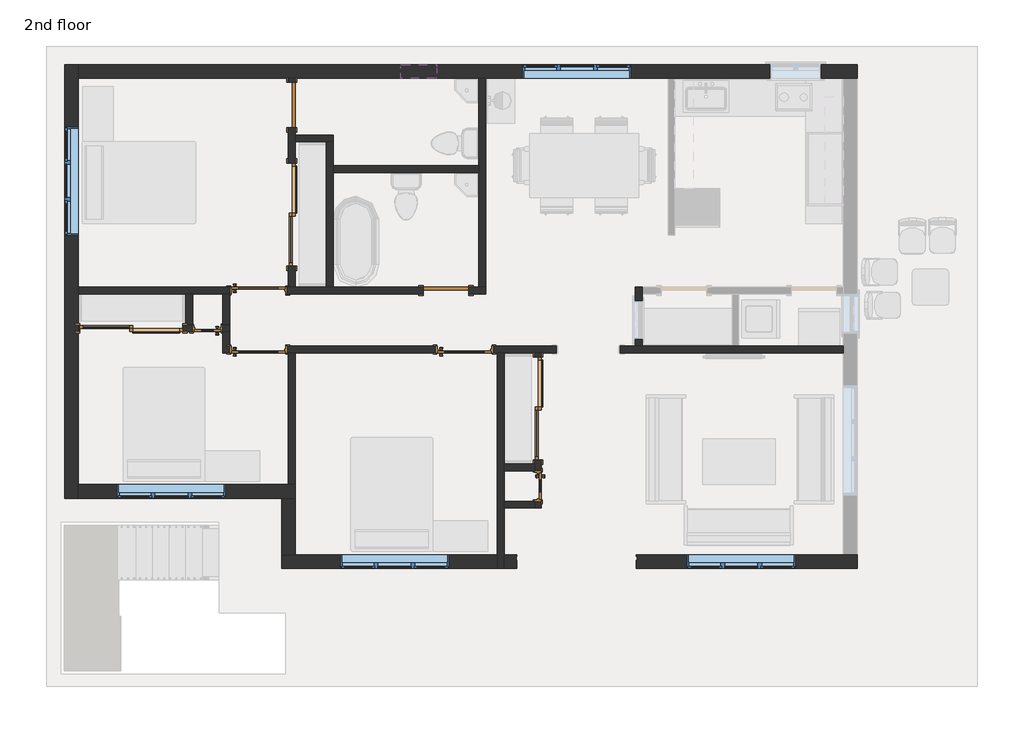
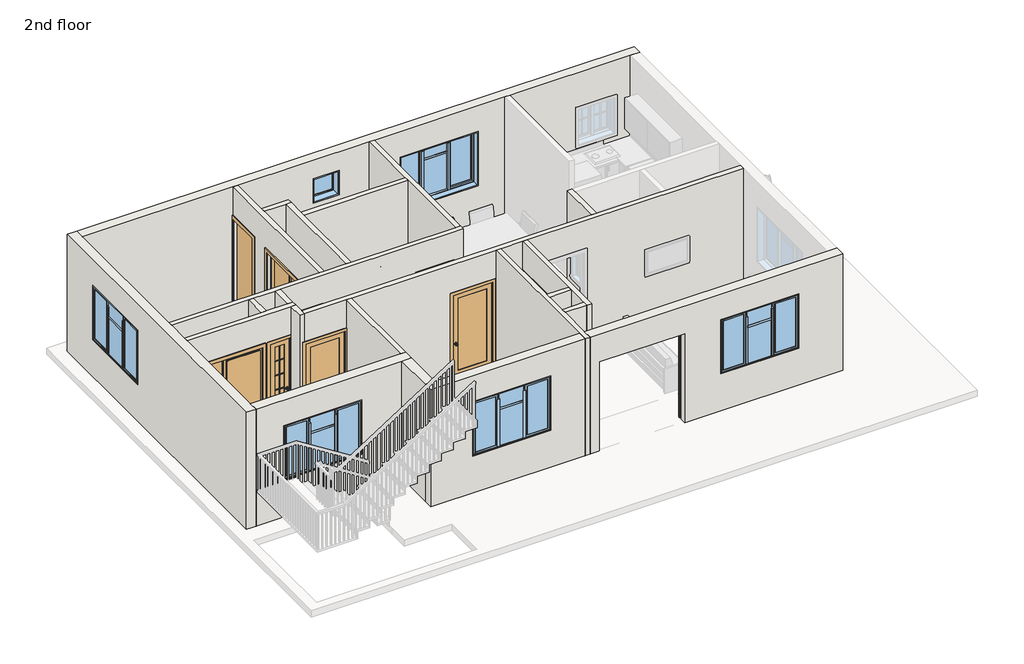
# One storey, part 1 of 4: 23 walls, 10 doors, 6 windows.
"""IFC4 building model written with IfcOpenShell, lengths in millimetres."""

from ifc_helpers import new_model, si_unit, frame, origin, place, context, project, spatial, polyline, outline, extrude, faceted_brep, transform, mapped, element, save
from components import door_505787c2, door_a3feeac7, door_3c6ab76a, door_ccf0cbd1, door_214872d5, door_78caadf7, window_80340324, window_7a1f68bc

model = new_model("IFC4")

# Units and contexts
model_context = context("Model", 3, world=origin())
ifc_project = project(units=[si_unit("LENGTHUNIT", "METRE", prefix="MILLI")], contexts=[model_context])

# Site, building, storey
site = spatial("IfcSite", under=ifc_project)
building = spatial("IfcBuilding", under=site)
storey = spatial("IfcBuildingStorey", under=building, Name="2nd floor", Elevation=7010.4)

# Doors
placement = place(None, origin())
door_shape = door_505787c2(model_context)
element("IfcDoor", 1, ObjectType="Door-Double-Sliding : 68\" x 84\"", at=placement, inside=storey, context=model_context, shape_type="MappedRepresentation", body=[
    mapped(door_shape, transform((-1350.0263529, 910.5161978, 7010.4), x_axis=(0.0, -1.0, 0.0), y_axis=(1.0, 0.0, 0.0), z_axis=(0.0, 0.0, 1.0))),
])
element("IfcDoor", 2, ObjectType="Door-Double-Sliding : 68\" x 84\"", at=placement, inside=storey, context=model_context, shape_type="MappedRepresentation", body=[
    mapped(door_shape, transform((-8046.1013529, 2383.7161978, 7010.4), x_axis=(-1.0, 0.0, 0.0), y_axis=(0.0, -1.0, 0.0), z_axis=(0.0, 0.0, 1.0))),
])
element("IfcDoor", 3, ObjectType="Door-Double-Sliding : 68\" x 84\"", at=placement, inside=storey, context=model_context, shape_type="MappedRepresentation", body=[
    mapped(door_shape, transform((-5477.5263529, 4168.0661978, 7010.4), x_axis=(0.0, -1.0, 0.0), y_axis=(1.0, 0.0, 0.0), z_axis=(0.0, 0.0, 1.0))),
])
door_2_shape = door_a3feeac7(model_context)
element("IfcDoor", 4, ObjectType="Door-Interior-Single-1_Panel-Wood : 36\" x 84\"", at=placement, inside=storey, context=model_context, shape_type="MappedRepresentation", body=[
    mapped(door_2_shape, transform((-5912.5013529, 1897.9411978, 7010.4), x_axis=(1.0, 0.0, 0.0), y_axis=(0.0, 1.0, 0.0), z_axis=(0.0, 0.0, 1.0))),
])
element("IfcDoor", 5, ObjectType="Door-Interior-Single-1_Panel-Wood : 36\" x 84\"", at=placement, inside=storey, context=model_context, shape_type="MappedRepresentation", body=[
    mapped(door_2_shape, transform((-2454.9263529, 1897.9411978, 7010.4), x_axis=(1.0, 0.0, 0.0), y_axis=(0.0, 1.0, 0.0), z_axis=(0.0, 0.0, 1.0))),
])
door_3_shape = door_3c6ab76a(model_context)
element("IfcDoor", 6, ObjectType="Door-Interior-Single-1_Panel-Wood : 36\" x 84\"", at=placement, inside=storey, context=model_context, shape_type="MappedRepresentation", body=[
    mapped(door_3_shape, transform((-5912.5013529, 2894.8911978, 7010.4), x_axis=(1.0, 0.0, 0.0), y_axis=(0.0, 1.0, 0.0), z_axis=(0.0, 0.0, 1.0))),
])
door_4_shape = door_ccf0cbd1(model_context)
element("IfcDoor", 7, ObjectType="Door-Interior-Single-Full Glass-Wood : 18\" x 84\"", at=placement, inside=storey, context=model_context, shape_type="MappedRepresentation", body=[
    mapped(door_4_shape, transform((-1219.8513529, -391.2338022, 7010.4), x_axis=(0.0, -1.0, 0.0), y_axis=(1.0, 0.0, 0.0), z_axis=(0.0, 0.0, 1.0))),
])
element("IfcDoor", 8, ObjectType="Door-Interior-Single-Full Glass-Wood : 18\" x 84\"", at=placement, inside=storey, context=model_context, shape_type="MappedRepresentation", body=[
    mapped(door_4_shape, transform((-6766.5763529, 2253.5411978, 7010.4), x_axis=(-1.0, 0.0, 0.0), y_axis=(0.0, -1.0, 0.0), z_axis=(0.0, 0.0, 1.0))),
])
door_5_shape = door_214872d5(model_context)
element("IfcDoor", 9, ObjectType="Single-Flush : 30\" x 84\"", at=placement, inside=storey, context=model_context, shape_type="MappedRepresentation", body=[
    mapped(door_5_shape, transform((-2766.0763529, 2891.7161978, 7010.4), x_axis=(1.0, 0.0, 0.0), y_axis=(0.0, 1.0, 0.0), z_axis=(0.0, 0.0, 1.0))),
])
door_6_shape = door_78caadf7(model_context)
element("IfcDoor", 10, ObjectType="Single-Flush : 30\" x 84\"", at=placement, inside=storey, context=model_context, shape_type="MappedRepresentation", body=[
    mapped(door_6_shape, transform((-5350.5263529, 6006.3911978, 7010.4), x_axis=(0.0, 1.0, 0.0), y_axis=(-1.0, 0.0, 0.0), z_axis=(0.0, 0.0, 1.0))),
])

# Walls
element("IfcWall", 11, ObjectType="Generic - 4.5\"", at=placement, inside=storey, context=model_context, shape_type="Brep", body=[
    faceted_brep([(-5407.6763529, 6454.0661978, 7010.4), (-5407.6763529, 6387.3911978, 7010.4), (-5407.6763529, 6387.3911978, 9144.0), (-5407.6763529, 5625.3911978, 9144.0), (-5407.6763529, 5625.3911978, 7010.4), (-5407.6763529, 5031.6661978, 7010.4), (-5407.6763529, 5031.6661978, 9144.0), (-5407.6763529, 3304.4661978, 9144.0), (-5407.6763529, 3304.4661978, 7010.4), (-5407.6763529, 2948.8661978, 7010.4), (-5407.6763529, 2948.8661978, 9906.0), (-5407.6763529, 6454.0661978, 9906.0), (-5293.3763529, 6387.3911978, 9144.0), (-5293.3763529, 6387.3911978, 7010.4), (-5293.3763529, 6454.0661978, 7010.4), (-5293.3763529, 6454.0661978, 9906.0), (-5293.3763529, 5501.5661978, 9906.0), (-5293.3763529, 5387.2661978, 9906.0), (-5293.3763529, 2948.8661978, 9906.0), (-5293.3763529, 2948.8661978, 7010.4), (-5293.3763529, 3304.4661978, 7010.4), (-5293.3763529, 3304.4661978, 9144.0), (-5293.3763529, 5031.6661978, 9144.0), (-5293.3763529, 5031.6661978, 7010.4), (-5293.3763529, 5387.2661978, 7010.4), (-5293.3763529, 5501.5661978, 7010.4), (-5293.3763529, 5625.3911978, 7010.4), (-5293.3763529, 5625.3911978, 9144.0)], [[[0, 1, 2, 3, 4, 5, 6, 7, 8, 9, 10, 11]], [[12, 13, 14, 15, 16, 17, 18, 19, 20, 21, 22, 23, 24, 25, 26, 27]], [[9, 8, 20, 19]], [[14, 13, 1, 0]], [[26, 25, 24, 23, 5, 4]], [[11, 10, 18, 17, 16, 15]], [[0, 11, 15, 14]], [[10, 9, 19, 18]], [[23, 22, 6, 5]], [[21, 20, 8, 7]], [[22, 21, 7, 6]], [[2, 1, 13, 12]], [[3, 2, 12, 27]], [[4, 3, 27, 26]]]),
])
element("IfcWall", 12, ObjectType="Generic - 4.5\"", at=placement, inside=storey, context=model_context, shape_type="Brep", body=[
    faceted_brep([(-2099.3263529, 2948.8661978, 7010.4), (-2213.6263529, 2948.8661978, 7010.4), (-2385.0763529, 2948.8661978, 7010.4), (-2385.0763529, 2948.8661978, 9144.0), (-3147.0763529, 2948.8661978, 9144.0), (-3147.0763529, 2948.8661978, 7010.4), (-4658.3763529, 2948.8661978, 7010.4), (-4772.6763529, 2948.8661978, 7010.4), (-5293.3763529, 2948.8661978, 7010.4), (-5407.6763529, 2948.8661978, 7010.4), (-5429.9013529, 2948.8661978, 7010.4), (-5429.9013529, 2948.8661978, 9169.4), (-6395.1013529, 2948.8661978, 9169.4), (-6395.1013529, 2948.8661978, 7010.4), (-8931.9263529, 2948.8661978, 7010.4), (-8931.9263529, 2948.8661978, 9906.0), (-5407.6763529, 2948.8661978, 9906.0), (-5293.3763529, 2948.8661978, 9906.0), (-4772.6763529, 2948.8661978, 9906.0), (-4658.3763529, 2948.8661978, 9906.0), (-2213.6263529, 2948.8661978, 9906.0), (-2099.3263529, 2948.8661978, 9906.0), (-2385.0763529, 2834.5661978, 9144.0), (-2385.0763529, 2834.5661978, 7010.4), (-2099.3263529, 2834.5661978, 7010.4), (-2099.3263529, 2834.5661978, 9906.0), (-6391.9263529, 2834.5661978, 9906.0), (-6506.2263529, 2834.5661978, 9906.0), (-7014.2263529, 2834.5661978, 9906.0), (-7128.5263529, 2834.5661978, 9906.0), (-8931.9263529, 2834.5661978, 9906.0), (-8931.9263529, 2834.5661978, 7010.4), (-7128.5263529, 2834.5661978, 7010.4), (-7014.2263529, 2834.5661978, 7010.4), (-6506.2263529, 2834.5661978, 7010.4), (-6395.1013529, 2834.5661978, 7010.4), (-6395.1013529, 2834.5661978, 9169.4), (-5429.9013529, 2834.5661978, 9169.4), (-5429.9013529, 2834.5661978, 7010.4), (-3147.0763529, 2834.5661978, 7010.4), (-3147.0763529, 2834.5661978, 9144.0)], [[[0, 1, 2, 3, 4, 5, 6, 7, 8, 9, 10, 11, 12, 13, 14, 15, 16, 17, 18, 19, 20, 21]], [[22, 23, 24, 25, 26, 27, 28, 29, 30, 31, 32, 33, 34, 35, 36, 37, 38, 39, 40]], [[31, 14, 13, 35, 34, 33, 32]], [[39, 38, 10, 9, 8, 7, 6, 5]], [[24, 23, 2, 1, 0]], [[21, 20, 19, 18, 17, 16, 15, 30, 29, 28, 27, 26, 25]], [[15, 14, 31, 30]], [[0, 21, 25, 24]], [[37, 11, 10, 38]], [[11, 37, 36, 12]], [[12, 36, 35, 13]], [[3, 2, 23, 22]], [[4, 3, 22, 40]], [[5, 4, 40, 39]]]),
])
element("IfcWall", 13, ObjectType="Generic - 4.5\"", at=placement, inside=storey, context=model_context, shape_type="Brep", body=[
    faceted_brep([(-8931.9263529, 2199.5661978, 7010.4), (-8909.7013529, 2199.5661978, 7010.4), (-8909.7013529, 2199.5661978, 9144.0), (-7182.5013529, 2199.5661978, 9144.0), (-7182.5013529, 2199.5661978, 7010.4), (-7020.5763529, 2199.5661978, 7010.4), (-7020.5763529, 2199.5661978, 9169.4), (-6512.5763529, 2199.5661978, 9169.4), (-6512.5763529, 2199.5661978, 7010.4), (-6506.2263529, 2199.5661978, 7010.4), (-6391.9263529, 2199.5661978, 7010.4), (-6391.9263529, 2199.5661978, 9906.0), (-6506.2263529, 2199.5661978, 9906.0), (-8931.9263529, 2199.5661978, 9906.0), (-8909.7013529, 2313.8661978, 9144.0), (-8909.7013529, 2313.8661978, 7010.4), (-8931.9263529, 2313.8661978, 7010.4), (-8931.9263529, 2313.8661978, 9906.0), (-7128.5263529, 2313.8661978, 9906.0), (-7014.2263529, 2313.8661978, 9906.0), (-6506.2263529, 2313.8661978, 9906.0), (-6391.9263529, 2313.8661978, 9906.0), (-6391.9263529, 2313.8661978, 7010.4), (-6506.2263529, 2313.8661978, 7010.4), (-6512.5763529, 2313.8661978, 7010.4), (-6512.5763529, 2313.8661978, 9169.4), (-7020.5763529, 2313.8661978, 9169.4), (-7020.5763529, 2313.8661978, 7010.4), (-7128.5263529, 2313.8661978, 7010.4), (-7182.5013529, 2313.8661978, 7010.4), (-7182.5013529, 2313.8661978, 9144.0)], [[[0, 1, 2, 3, 4, 5, 6, 7, 8, 9, 10, 11, 12, 13]], [[14, 15, 16, 17, 18, 19, 20, 21, 22, 23, 24, 25, 26, 27, 28, 29, 30]], [[22, 10, 9, 8, 24, 23]], [[16, 15, 1, 0]], [[29, 28, 27, 5, 4]], [[13, 12, 11, 21, 20, 19, 18, 17]], [[0, 13, 17, 16]], [[11, 10, 22, 21]], [[26, 6, 5, 27]], [[6, 26, 25, 7]], [[7, 25, 24, 8]], [[4, 3, 30, 29]], [[2, 1, 15, 14]], [[3, 2, 14, 30]]]),
])
element("IfcWall", 14, ObjectType="Generic - 4.5\"", at=placement, inside=storey, context=model_context, shape_type="Brep", body=[
    faceted_brep([(-7014.2263529, 2313.8661978, 7010.4), (-7014.2263529, 2834.5661978, 7010.4), (-7014.2263529, 2834.5661978, 9906.0), (-7014.2263529, 2313.8661978, 9906.0), (-7128.5263529, 2313.8661978, 7010.4), (-7128.5263529, 2313.8661978, 9906.0), (-7128.5263529, 2834.5661978, 9906.0), (-7128.5263529, 2834.5661978, 7010.4), (-7020.5763529, 2313.8661978, 7010.4)], [[[0, 1, 2, 3]], [[4, 5, 6, 7]], [[1, 0, 8, 4, 7]], [[3, 2, 6, 5]], [[0, 3, 5, 4, 8]], [[2, 1, 7, 6]]]),
])
element("IfcWall", 15, ObjectType="Generic - 4.5\"", at=placement, inside=storey, context=model_context, shape_type="Brep", body=[
    faceted_brep([(-6391.9263529, 2313.8661978, 7010.4), (-6391.9263529, 2834.5661978, 7010.4), (-6391.9263529, 2834.5661978, 9906.0), (-6391.9263529, 2313.8661978, 9906.0), (-6506.2263529, 2313.8661978, 7010.4), (-6506.2263529, 2313.8661978, 9906.0), (-6506.2263529, 2834.5661978, 9906.0), (-6506.2263529, 2834.5661978, 7010.4), (-6395.1013529, 2834.5661978, 7010.4)], [[[0, 1, 2, 3]], [[4, 5, 6, 7]], [[1, 0, 4, 7, 8]], [[3, 2, 6, 5]], [[0, 3, 5, 4]], [[2, 1, 8, 7, 6]]]),
])
element("IfcWall", 16, ObjectType="Generic - 4.5\"", at=placement, inside=storey, context=model_context, shape_type="SweptSolid", body=[
    extrude(outline(polyline([(-5293.3763529, 1843.9661978), (-5293.3763529, -365.8338022), (-5407.6763529, -365.8338022), (-5407.6763529, 1843.9661978), (-5293.3763529, 1843.9661978)])), frame((0.0, 0.0, 7010.4), z_axis=(0.0, 0.0, 1.0), x_axis=(1.0, 0.0, 0.0)), (0.0, 0.0, 1.0), 2895.6),
])
element("IfcWall", 17, ObjectType="Generic - 4.5\"", at=placement, inside=storey, context=model_context, shape_type="Brep", body=[
    faceted_brep([(-6506.2263529, 2199.5661978, 7010.4), (-6506.2263529, 1843.9661978, 7010.4), (-6506.2263529, 1843.9661978, 9906.0), (-6506.2263529, 2199.5661978, 9906.0), (-6391.9263529, 2199.5661978, 9906.0), (-6391.9263529, 1958.2661978, 9906.0), (-6391.9263529, 1843.9661978, 9906.0), (-6391.9263529, 1843.9661978, 9169.4), (-6391.9263529, 1958.2661978, 9169.4), (-6391.9263529, 1958.2661978, 7010.4), (-6391.9263529, 2199.5661978, 7010.4), (-6395.1013529, 1958.2661978, 7010.4), (-6395.1013529, 1843.9661978, 7010.4), (-6395.1013529, 1843.9661978, 9169.4), (-6395.1013529, 1958.2661978, 9169.4)], [[[0, 1, 2, 3]], [[4, 5, 6, 7, 8, 9, 10]], [[1, 0, 10, 9, 11, 12]], [[3, 2, 6, 5, 4]], [[0, 3, 4, 10]], [[2, 1, 12, 13, 7, 6]], [[14, 11, 9, 8]], [[13, 14, 8, 7]], [[11, 14, 13, 12]]]),
])
element("IfcWall", 18, ObjectType="Generic - 4.5\"", at=placement, inside=storey, context=model_context, shape_type="Brep", body=[
    faceted_brep([(-1972.3263529, 1843.9661978, 7010.4), (-1902.4763529, 1843.9661978, 7010.4), (-1788.1763529, 1843.9661978, 7010.4), (-1280.1763529, 1843.9661978, 7010.4), (-1165.8763529, 1843.9661978, 7010.4), (-911.8763529, 1843.9661978, 7010.4), (-911.8763529, 1843.9661978, 9144.0), (154.9236471, 1843.9661978, 9144.0), (154.9236471, 1843.9661978, 7010.4), (3901.4236471, 1843.9661978, 7010.4), (3901.4236471, 1843.9661978, 9906.0), (-1165.8763529, 1843.9661978, 9906.0), (-1280.1763529, 1843.9661978, 9906.0), (-1788.1763529, 1843.9661978, 9906.0), (-1902.4763529, 1843.9661978, 9906.0), (-5293.3763529, 1843.9661978, 9906.0), (-5407.6763529, 1843.9661978, 9906.0), (-6391.9263529, 1843.9661978, 9906.0), (-6391.9263529, 1843.9661978, 9169.4), (-5429.9013529, 1843.9661978, 9169.4), (-5429.9013529, 1843.9661978, 7010.4), (-5407.6763529, 1843.9661978, 7010.4), (-5293.3763529, 1843.9661978, 7010.4), (-2937.5263529, 1843.9661978, 7010.4), (-2937.5263529, 1843.9661978, 9169.4), (-1972.3263529, 1843.9661978, 9169.4), (-911.8763529, 1958.2661978, 9144.0), (-911.8763529, 1958.2661978, 7010.4), (-1972.3263529, 1958.2661978, 7010.4), (-1972.3263529, 1958.2661978, 9169.4), (-2937.5263529, 1958.2661978, 9169.4), (-2937.5263529, 1958.2661978, 7010.4), (-5429.9013529, 1958.2661978, 7010.4), (-5429.9013529, 1958.2661978, 9169.4), (-6391.9263529, 1958.2661978, 9169.4), (-6391.9263529, 1958.2661978, 9906.0), (408.9236471, 1958.2661978, 9906.0), (523.2236471, 1958.2661978, 9906.0), (2034.5236471, 1958.2661978, 9906.0), (2148.8236471, 1958.2661978, 9906.0), (3901.4236471, 1958.2661978, 9906.0), (3901.4236471, 1958.2661978, 7010.4), (2148.8236471, 1958.2661978, 7010.4), (2034.5236471, 1958.2661978, 7010.4), (523.2236471, 1958.2661978, 7010.4), (408.9236471, 1958.2661978, 7010.4), (154.9236471, 1958.2661978, 7010.4), (154.9236471, 1958.2661978, 9144.0)], [[[0, 1, 2, 3, 4, 5, 6, 7, 8, 9, 10, 11, 12, 13, 14, 15, 16, 17, 18, 19, 20, 21, 22, 23, 24, 25]], [[26, 27, 28, 29, 30, 31, 32, 33, 34, 35, 36, 37, 38, 39, 40, 41, 42, 43, 44, 45, 46, 47]], [[20, 32, 31, 23, 22, 21]], [[28, 27, 5, 4, 3, 2, 1, 0]], [[46, 45, 44, 43, 42, 41, 9, 8]], [[17, 16, 15, 14, 13, 12, 11, 10, 40, 39, 38, 37, 36, 35]], [[17, 35, 34, 18]], [[10, 9, 41, 40]], [[19, 18, 34, 33]], [[25, 29, 28, 0]], [[29, 25, 24, 30]], [[30, 24, 23, 31]], [[19, 33, 32, 20]], [[8, 7, 47, 46]], [[6, 5, 27, 26]], [[7, 6, 26, 47]]]),
])
element("IfcWall", 19, ObjectType="Generic - 4.5\"", at=placement, inside=storey, context=model_context, shape_type="Brep", body=[
    faceted_brep([(-1902.4763529, 1843.9661978, 7010.4), (-1902.4763529, -1546.9338022, 7010.4), (-1902.4763529, -1775.5338022, 7010.4), (-1902.4763529, -1775.5338022, 9906.0), (-1902.4763529, -1546.9338022, 9906.0), (-1902.4763529, 1843.9661978, 9906.0), (-1788.1763529, 1843.9661978, 7010.4), (-1788.1763529, 1843.9661978, 9906.0), (-1788.1763529, -22.9338022, 9906.0), (-1788.1763529, -137.2338022, 9906.0), (-1788.1763529, -645.2338022, 9906.0), (-1788.1763529, -759.5338022, 9906.0), (-1788.1763529, -1546.9338022, 9906.0), (-1788.1763529, -1775.5338022, 9906.0), (-1788.1763529, -1775.5338022, 7010.4), (-1788.1763529, -1546.9338022, 7010.4), (-1788.1763529, -759.5338022, 7010.4), (-1788.1763529, -645.2338022, 7010.4), (-1788.1763529, -137.2338022, 7010.4), (-1788.1763529, -22.9338022, 7010.4)], [[[0, 1, 2, 3, 4, 5]], [[6, 7, 8, 9, 10, 11, 12, 13, 14, 15, 16, 17, 18, 19]], [[2, 1, 0, 6, 19, 18, 17, 16, 15, 14]], [[5, 4, 3, 13, 12, 11, 10, 9, 8, 7]], [[0, 5, 7, 6]], [[3, 2, 14, 13]]]),
])
element("IfcWall", 20, ObjectType="Generic - 4.5\"", at=placement, inside=storey, context=model_context, shape_type="Brep", body=[
    faceted_brep([(-1280.1763529, 46.9161978, 9144.0), (-1280.1763529, 46.9161978, 7010.4), (-1280.1763529, -22.9338022, 7010.4), (-1280.1763529, -137.2338022, 7010.4), (-1280.1763529, -137.2338022, 9169.4), (-1280.1763529, -645.2338022, 9169.4), (-1280.1763529, -645.2338022, 7010.4), (-1280.1763529, -759.5338022, 7010.4), (-1280.1763529, -759.5338022, 9906.0), (-1280.1763529, -645.2338022, 9906.0), (-1280.1763529, -137.2338022, 9906.0), (-1280.1763529, -22.9338022, 9906.0), (-1280.1763529, 1843.9661978, 9906.0), (-1280.1763529, 1843.9661978, 7010.4), (-1280.1763529, 1774.1161978, 7010.4), (-1280.1763529, 1774.1161978, 9144.0), (-1165.8763529, -137.2338022, 7010.4), (-1165.8763529, 46.9161978, 7010.4), (-1165.8763529, 46.9161978, 9144.0), (-1165.8763529, 1774.1161978, 9144.0), (-1165.8763529, 1774.1161978, 7010.4), (-1165.8763529, 1843.9661978, 7010.4), (-1165.8763529, 1843.9661978, 9906.0), (-1165.8763529, -759.5338022, 9906.0), (-1165.8763529, -759.5338022, 7010.4), (-1165.8763529, -645.2338022, 7010.4), (-1165.8763529, -645.2338022, 9169.4), (-1165.8763529, -137.2338022, 9169.4)], [[[0, 1, 2, 3, 4, 5, 6, 7, 8, 9, 10, 11, 12, 13, 14, 15]], [[16, 17, 18, 19, 20, 21, 22, 23, 24, 25, 26, 27]], [[24, 7, 6, 25]], [[14, 13, 21, 20]], [[3, 2, 1, 17, 16]], [[12, 11, 10, 9, 8, 23, 22]], [[13, 12, 22, 21]], [[8, 7, 24, 23]], [[5, 26, 25, 6]], [[26, 5, 4, 27]], [[27, 4, 3, 16]], [[20, 19, 15, 14]], [[18, 17, 1, 0]], [[19, 18, 0, 15]]]),
])
element("IfcWall", 21, ObjectType="Generic - 4.5\"", at=placement, inside=storey, context=model_context, shape_type="Brep", body=[
    faceted_brep([(-1280.1763529, -22.9338022, 7010.4), (-1788.1763529, -22.9338022, 7010.4), (-1788.1763529, -22.9338022, 9906.0), (-1280.1763529, -22.9338022, 9906.0), (-1280.1763529, -137.2338022, 7010.4), (-1280.1763529, -137.2338022, 9169.4), (-1280.1763529, -137.2338022, 9906.0), (-1788.1763529, -137.2338022, 9906.0), (-1788.1763529, -137.2338022, 7010.4)], [[[0, 1, 2, 3]], [[4, 5, 6, 7, 8]], [[1, 0, 4, 8]], [[3, 2, 7, 6]], [[0, 3, 6, 5, 4]], [[2, 1, 8, 7]]]),
])
element("IfcWall", 22, ObjectType="Generic - 4.5\"", at=placement, inside=storey, context=model_context, shape_type="Brep", body=[
    faceted_brep([(-1280.1763529, -645.2338022, 7010.4), (-1788.1763529, -645.2338022, 7010.4), (-1788.1763529, -645.2338022, 9906.0), (-1280.1763529, -645.2338022, 9906.0), (-1280.1763529, -645.2338022, 9169.4), (-1280.1763529, -759.5338022, 7010.4), (-1280.1763529, -759.5338022, 9906.0), (-1788.1763529, -759.5338022, 9906.0), (-1788.1763529, -759.5338022, 7010.4)], [[[0, 1, 2, 3, 4]], [[5, 6, 7, 8]], [[1, 0, 5, 8]], [[3, 2, 7, 6]], [[0, 4, 3, 6, 5]], [[2, 1, 8, 7]]]),
])
element("IfcWall", 23, ObjectType="Generic - 4.5\"", at=placement, inside=storey, context=model_context, shape_type="Brep", body=[
    faceted_brep([(-2099.3263529, 2948.8661978, 7010.4), (-2099.3263529, 6454.0661978, 7010.4), (-2099.3263529, 6454.0661978, 9906.0), (-2099.3263529, 2948.8661978, 9906.0), (-2213.6263529, 2948.8661978, 7010.4), (-2213.6263529, 2948.8661978, 9906.0), (-2213.6263529, 4872.9161978, 9906.0), (-2213.6263529, 4987.2161978, 9906.0), (-2213.6263529, 6454.0661978, 9906.0), (-2213.6263529, 6454.0661978, 7010.4), (-2213.6263529, 4987.2161978, 7010.4), (-2213.6263529, 4872.9161978, 7010.4)], [[[0, 1, 2, 3]], [[4, 5, 6, 7, 8, 9, 10, 11]], [[1, 0, 4, 11, 10, 9]], [[3, 2, 8, 7, 6, 5]], [[2, 1, 9, 8]], [[0, 3, 5, 4]]]),
])
element("IfcWall", 24, ObjectType="Generic - 4.5\"", at=placement, inside=storey, context=model_context, shape_type="Brep", body=[
    faceted_brep([(-5293.3763529, 5387.2661978, 7010.4), (-4772.6763529, 5387.2661978, 7010.4), (-4658.3763529, 5387.2661978, 7010.4), (-4658.3763529, 5387.2661978, 9906.0), (-4772.6763529, 5387.2661978, 9906.0), (-5293.3763529, 5387.2661978, 9906.0), (-5293.3763529, 5501.5661978, 7010.4), (-5293.3763529, 5501.5661978, 9906.0), (-4658.3763529, 5501.5661978, 9906.0), (-4658.3763529, 5501.5661978, 7010.4)], [[[0, 1, 2, 3, 4, 5]], [[6, 7, 8, 9]], [[2, 1, 0, 6, 9]], [[5, 4, 3, 8, 7]], [[0, 5, 7, 6]], [[3, 2, 9, 8]]]),
])
element("IfcWall", 25, ObjectType="Generic - 4.5\"", at=placement, inside=storey, context=model_context, shape_type="Brep", body=[
    faceted_brep([(-4772.6763529, 5387.2661978, 7010.4), (-4772.6763529, 2948.8661978, 7010.4), (-4772.6763529, 2948.8661978, 9906.0), (-4772.6763529, 5387.2661978, 9906.0), (-4658.3763529, 5387.2661978, 7010.4), (-4658.3763529, 5387.2661978, 9906.0), (-4658.3763529, 4987.2161978, 9906.0), (-4658.3763529, 4872.9161978, 9906.0), (-4658.3763529, 2948.8661978, 9906.0), (-4658.3763529, 2948.8661978, 7010.4), (-4658.3763529, 4872.9161978, 7010.4), (-4658.3763529, 4987.2161978, 7010.4)], [[[0, 1, 2, 3]], [[4, 5, 6, 7, 8, 9, 10, 11]], [[1, 0, 4, 11, 10, 9]], [[3, 2, 8, 7, 6, 5]], [[0, 3, 5, 4]], [[2, 1, 9, 8]]]),
])
element("IfcWall", 26, ObjectType="Generic - 4.5\"", at=placement, inside=storey, context=model_context, shape_type="SweptSolid", body=[
    extrude(outline(polyline([(-4658.3763529, 4987.2161978), (-2213.6263529, 4987.2161978), (-2213.6263529, 4872.9161978), (-4658.3763529, 4872.9161978), (-4658.3763529, 4987.2161978)])), frame((0.0, 0.0, 7010.4), z_axis=(0.0, 0.0, 1.0), x_axis=(1.0, 0.0, 0.0)), (0.0, 0.0, 1.0), 2895.6),
])
element("IfcWall", 27, ObjectType="Generic - 4.5\"", at=placement, inside=storey, context=model_context, shape_type="Brep", body=[
    faceted_brep([(523.2236471, 1958.2661978, 7010.4), (523.2236471, 2834.5661978, 7010.4), (523.2236471, 2948.8661978, 7010.4), (523.2236471, 2948.8661978, 9906.0), (523.2236471, 2834.5661978, 9906.0), (523.2236471, 1958.2661978, 9906.0), (523.2236471, 2726.6161978, 8991.6), (523.2236471, 2726.6161978, 7924.8), (523.2236471, 2066.2161978, 7924.8), (523.2236471, 2066.2161978, 8991.6), (408.9236471, 1958.2661978, 7010.4), (408.9236471, 1958.2661978, 9906.0), (408.9236471, 2948.8661978, 9906.0), (408.9236471, 2948.8661978, 7010.4), (408.9236471, 2726.6161978, 8991.6), (408.9236471, 2066.2161978, 8991.6), (408.9236471, 2066.2161978, 7924.8), (408.9236471, 2726.6161978, 7924.8)], [[[0, 1, 2, 3, 4, 5], [6, 7, 8, 9]], [[10, 11, 12, 13], [14, 15, 16, 17]], [[2, 1, 0, 10, 13]], [[5, 4, 3, 12, 11]], [[0, 5, 11, 10]], [[3, 2, 13, 12]], [[7, 6, 14, 17]], [[8, 7, 17, 16]], [[9, 8, 16, 15]], [[6, 9, 15, 14]]]),
])
element("IfcWall", 28, ObjectType="Generic - 9\"", at=placement, inside=storey, context=model_context, shape_type="Brep", body=[
    faceted_brep([(-9160.5263529, 6682.6661978, 7010.4), (-9160.5263529, -594.4338022, 7010.4), (-9160.5263529, -594.4338022, 9906.0), (-9160.5263529, 6682.6661978, 9906.0), (-9160.5263529, 5644.4411978, 9271.0), (-9160.5263529, 3815.6411978, 9271.0), (-9160.5263529, 3815.6411978, 7924.8), (-9160.5263529, 5644.4411978, 7924.8), (-8931.9263529, 6682.6661978, 7010.4), (-8931.9263529, 6682.6661978, 9906.0), (-8931.9263529, 6454.0661978, 9906.0), (-8931.9263529, 2948.8661978, 9906.0), (-8931.9263529, 2834.5661978, 9906.0), (-8931.9263529, 2313.8661978, 9906.0), (-8931.9263529, 2199.5661978, 9906.0), (-8931.9263529, -365.8338022, 9906.0), (-8931.9263529, -594.4338022, 9906.0), (-8931.9263529, -594.4338022, 7010.4), (-8931.9263529, -365.8338022, 7010.4), (-8931.9263529, 2199.5661978, 7010.4), (-8931.9263529, 2313.8661978, 7010.4), (-8931.9263529, 2834.5661978, 7010.4), (-8931.9263529, 2948.8661978, 7010.4), (-8931.9263529, 6454.0661978, 7010.4), (-8931.9263529, 5644.4411978, 9271.0), (-8931.9263529, 5644.4411978, 7924.8), (-8931.9263529, 3815.6411978, 7924.8), (-8931.9263529, 3815.6411978, 9271.0)], [[[0, 1, 2, 3], [4, 5, 6, 7]], [[8, 9, 10, 11, 12, 13, 14, 15, 16, 17, 18, 19, 20, 21, 22, 23], [24, 25, 26, 27]], [[1, 0, 8, 23, 22, 21, 20, 19, 18, 17]], [[3, 2, 16, 15, 14, 13, 12, 11, 10, 9]], [[0, 3, 9, 8]], [[2, 1, 17, 16]], [[25, 24, 4, 7]], [[26, 25, 7, 6]], [[27, 26, 6, 5]], [[24, 27, 5, 4]]]),
])
element("IfcWall", 29, ObjectType="Generic - 9\"", at=placement, inside=storey, context=model_context, shape_type="Brep", body=[
    faceted_brep([(-8931.9263529, 6454.0661978, 7010.4), (-5407.6763529, 6454.0661978, 7010.4), (-5293.3763529, 6454.0661978, 7010.4), (-2213.6263529, 6454.0661978, 7010.4), (-2099.3263529, 6454.0661978, 7010.4), (961.3736471, 6454.0661978, 7010.4), (1075.6736471, 6454.0661978, 7010.4), (3901.4236471, 6454.0661978, 7010.4), (4130.0236471, 6454.0661978, 7010.4), (4130.0236471, 6454.0661978, 9906.0), (3901.4236471, 6454.0661978, 9906.0), (1075.6736471, 6454.0661978, 9906.0), (961.3736471, 6454.0661978, 9906.0), (-2099.3263529, 6454.0661978, 9906.0), (-2213.6263529, 6454.0661978, 9906.0), (-5293.3763529, 6454.0661978, 9906.0), (-5407.6763529, 6454.0661978, 9906.0), (-8931.9263529, 6454.0661978, 9906.0), (3533.1236471, 6454.0661978, 9017.0), (3533.1236471, 6454.0661978, 8102.6), (2669.5236471, 6454.0661978, 8102.6), (2669.5236471, 6454.0661978, 9017.0), (345.4236471, 6454.0661978, 9271.0), (345.4236471, 6454.0661978, 7924.8), (-1483.3763529, 6454.0661978, 7924.8), (-1483.3763529, 6454.0661978, 9271.0), (-2918.4763529, 6454.0661978, 9448.8), (-2918.4763529, 6454.0661978, 8839.2), (-3528.0763529, 6454.0661978, 8839.2), (-3528.0763529, 6454.0661978, 9448.8), (-8931.9263529, 6682.6661978, 7010.4), (-8931.9263529, 6682.6661978, 9906.0), (4130.0236471, 6682.6661978, 9906.0), (4130.0236471, 6682.6661978, 7010.4), (3533.1236471, 6682.6661978, 9017.0), (2669.5236471, 6682.6661978, 9017.0), (2669.5236471, 6682.6661978, 8102.6), (3533.1236471, 6682.6661978, 8102.6), (345.4236471, 6682.6661978, 9271.0), (-1483.3763529, 6682.6661978, 9271.0), (-1483.3763529, 6682.6661978, 7924.8), (345.4236471, 6682.6661978, 7924.8), (-2918.4763529, 6682.6661978, 9448.8), (-3528.0763529, 6682.6661978, 9448.8), (-3528.0763529, 6682.6661978, 8839.2), (-2918.4763529, 6682.6661978, 8839.2)], [[[0, 1, 2, 3, 4, 5, 6, 7, 8, 9, 10, 11, 12, 13, 14, 15, 16, 17], [18, 19, 20, 21], [22, 23, 24, 25], [26, 27, 28, 29]], [[30, 31, 32, 33], [34, 35, 36, 37], [38, 39, 40, 41], [42, 43, 44, 45]], [[8, 7, 6, 5, 4, 3, 2, 1, 0, 30, 33]], [[17, 16, 15, 14, 13, 12, 11, 10, 9, 32, 31]], [[0, 17, 31, 30]], [[9, 8, 33, 32]], [[19, 18, 34, 37]], [[20, 19, 37, 36]], [[21, 20, 36, 35]], [[18, 21, 35, 34]], [[23, 22, 38, 41]], [[24, 23, 41, 40]], [[25, 24, 40, 39]], [[22, 25, 39, 38]], [[27, 26, 42, 45]], [[28, 27, 45, 44]], [[29, 28, 44, 43]], [[26, 29, 43, 42]]]),
])
element("IfcWall", 30, ObjectType="Generic - 9\"", at=placement, inside=storey, context=model_context, shape_type="Brep", body=[
    faceted_brep([(-8931.9263529, -594.4338022, 7010.4), (-5521.9763529, -594.4338022, 7010.4), (-5293.3763529, -594.4338022, 7010.4), (-5293.3763529, -594.4338022, 9906.0), (-5521.9763529, -594.4338022, 9906.0), (-8931.9263529, -594.4338022, 9906.0), (-8284.2263529, -594.4338022, 9271.0), (-6455.4263529, -594.4338022, 9271.0), (-6455.4263529, -594.4338022, 7924.8), (-8284.2263529, -594.4338022, 7924.8), (-8931.9263529, -365.8338022, 7010.4), (-8931.9263529, -365.8338022, 9906.0), (-5407.6763529, -365.8338022, 9906.0), (-5293.3763529, -365.8338022, 9906.0), (-5293.3763529, -365.8338022, 7010.4), (-5407.6763529, -365.8338022, 7010.4), (-8284.2263529, -365.8338022, 9271.0), (-8284.2263529, -365.8338022, 7924.8), (-6455.4263529, -365.8338022, 7924.8), (-6455.4263529, -365.8338022, 9271.0)], [[[0, 1, 2, 3, 4, 5], [6, 7, 8, 9]], [[10, 11, 12, 13, 14, 15], [16, 17, 18, 19]], [[2, 1, 0, 10, 15, 14]], [[5, 4, 3, 13, 12, 11]], [[3, 2, 14, 13]], [[0, 5, 11, 10]], [[17, 16, 6, 9]], [[18, 17, 9, 8]], [[19, 18, 8, 7]], [[16, 19, 7, 6]]]),
])
element("IfcWall", 31, ObjectType="Generic - 9\"", at=placement, inside=storey, context=model_context, shape_type="Brep", body=[
    faceted_brep([(-1902.4763529, -1546.9338022, 7010.4), (-5293.3763529, -1546.9338022, 7010.4), (-5521.9763529, -1546.9338022, 7010.4), (-5521.9763529, -1546.9338022, 9906.0), (-5293.3763529, -1546.9338022, 9906.0), (-1902.4763529, -1546.9338022, 9906.0), (-4540.9013529, -1546.9338022, 9271.0), (-4540.9013529, -1546.9338022, 7924.8), (-2712.1013529, -1546.9338022, 7924.8), (-2712.1013529, -1546.9338022, 9271.0), (-1902.4763529, -1775.5338022, 7010.4), (-1902.4763529, -1775.5338022, 9906.0), (-5521.9763529, -1775.5338022, 9906.0), (-5521.9763529, -1775.5338022, 7010.4), (-4540.9013529, -1775.5338022, 9271.0), (-2712.1013529, -1775.5338022, 9271.0), (-2712.1013529, -1775.5338022, 7924.8), (-4540.9013529, -1775.5338022, 7924.8)], [[[0, 1, 2, 3, 4, 5], [6, 7, 8, 9]], [[10, 11, 12, 13], [14, 15, 16, 17]], [[2, 1, 0, 10, 13]], [[5, 4, 3, 12, 11]], [[0, 5, 11, 10]], [[3, 2, 13, 12]], [[7, 6, 14, 17]], [[8, 7, 17, 16]], [[9, 8, 16, 15]], [[6, 9, 15, 14]]]),
])
element("IfcWall", 32, ObjectType="Generic - 9\"", at=placement, inside=storey, context=model_context, shape_type="SweptSolid", body=[
    extrude(outline(polyline([(-5521.9763529, -1546.9338022), (-5521.9763529, -594.4338022), (-5293.3763529, -594.4338022), (-5293.3763529, -1546.9338022), (-5521.9763529, -1546.9338022)])), frame((0.0, 0.0, 7010.4), z_axis=(0.0, 0.0, 1.0), x_axis=(1.0, 0.0, 0.0)), (0.0, 0.0, 1.0), 2895.6),
])
element("IfcWall", 33, ObjectType="Generic - 9\"", at=placement, inside=storey, context=model_context, shape_type="Brep", body=[
    faceted_brep([(4130.0236471, -1775.5338022, 9906.0), (-1788.1763529, -1775.5338022, 9906.0), (-1788.1763529, -1775.5338022, 7010.4), (-1575.3263529, -1775.5338022, 7010.4), (-1575.3263529, -1775.5338022, 9219.4), (424.6736471, -1775.5338022, 9219.4), (424.6736471, -1775.5338022, 7010.4), (4130.0236471, -1775.5338022, 7010.4), (1272.5236471, -1775.5338022, 9271.0), (3101.3236471, -1775.5338022, 9271.0), (3101.3236471, -1775.5338022, 7924.8), (1272.5236471, -1775.5338022, 7924.8), (-1788.1763529, -1546.9338022, 9906.0), (3901.4236471, -1546.9338022, 9906.0), (4130.0236471, -1546.9338022, 9906.0), (4130.0236471, -1546.9338022, 7010.4), (3901.4236471, -1546.9338022, 7010.4), (424.6736471, -1546.9338022, 7010.4), (424.6736471, -1546.9338022, 9219.4), (-1575.3263529, -1546.9338022, 9219.4), (-1575.3263529, -1546.9338022, 7010.4), (-1788.1763529, -1546.9338022, 7010.4), (1272.5236471, -1546.9338022, 9271.0), (1272.5236471, -1546.9338022, 7924.8), (3101.3236471, -1546.9338022, 7924.8), (3101.3236471, -1546.9338022, 9271.0), (-1575.3263529, -1566.9338022, 7010.4), (-1590.3263529, -1566.9338022, 7010.4), (-1590.3263529, -1636.9338022, 7010.4), (-1575.3263529, -1636.9338022, 7010.4), (424.6736471, -1636.9338022, 7010.4), (439.6736471, -1636.9338022, 7010.4), (439.6736471, -1566.9338022, 7010.4), (424.6736471, -1566.9338022, 7010.4), (424.6736471, -1566.9338022, 9219.4), (-1575.3263529, -1566.9338022, 9219.4), (-1575.3263529, -1636.9338022, 9219.4), (424.6736471, -1636.9338022, 9219.4), (-1590.3263529, -1636.9338022, 9234.4), (439.6736471, -1636.9338022, 9234.4), (439.6736471, -1566.9338022, 9234.4), (-1590.3263529, -1566.9338022, 9234.4)], [[[0, 1, 2, 3, 4, 5, 6, 7], [8, 9, 10, 11]], [[12, 13, 14, 15, 16, 17, 18, 19, 20, 21], [22, 23, 24, 25]], [[2, 21, 20, 26, 27, 28, 29, 3]], [[15, 7, 6, 30, 31, 32, 33, 17, 16]], [[1, 0, 14, 13, 12]], [[2, 1, 12, 21]], [[0, 7, 15, 14]], [[34, 35, 19, 18]], [[36, 37, 5, 4]], [[29, 36, 4, 3]], [[37, 30, 6, 5]], [[37, 36, 29, 28, 38, 39, 31, 30]], [[31, 39, 40, 32]], [[35, 34, 33, 32, 40, 41, 27, 26]], [[33, 34, 18, 17]], [[35, 26, 20, 19]], [[38, 28, 27, 41]], [[39, 38, 41, 40]], [[23, 22, 8, 11]], [[24, 23, 11, 10]], [[25, 24, 10, 9]], [[22, 25, 9, 8]]]),
])

# Windows
window_shape = window_80340324(model_context)
element("IfcWindow", 34, ObjectType="Fixed : 24\" x 24\"", at=placement, inside=storey, context=model_context, shape_type="MappedRepresentation", body=[
    mapped(window_shape, transform((-3185.1763529, 6568.3661978, 7924.8), x_axis=(1.0, 0.0, 0.0), y_axis=(0.0, 1.0, 0.0), z_axis=(0.0, 0.0, 1.0))),
])
window_2_shape = window_7a1f68bc(model_context)
element("IfcWindow", 35, ObjectType="Window-Casement-Triple-Middle-Transom : 72\" x 53\"", at=placement, inside=storey, context=model_context, shape_type="MappedRepresentation", body=[
    mapped(window_2_shape, transform((-3626.5013529, -1661.2338022, 7010.4), x_axis=(-1.0, 0.0, 0.0), y_axis=(0.0, -1.0, 0.0), z_axis=(0.0, 0.0, 1.0))),
])
element("IfcWindow", 36, ObjectType="Window-Casement-Triple-Middle-Transom : 72\" x 53\"", at=placement, inside=storey, context=model_context, shape_type="MappedRepresentation", body=[
    mapped(window_2_shape, transform((-7369.8263529, -480.1338022, 7010.4), x_axis=(-1.0, 0.0, 0.0), y_axis=(0.0, -1.0, 0.0), z_axis=(0.0, 0.0, 1.0))),
])
element("IfcWindow", 37, ObjectType="Window-Casement-Triple-Middle-Transom : 72\" x 53\"", at=placement, inside=storey, context=model_context, shape_type="MappedRepresentation", body=[
    mapped(window_2_shape, transform((-9046.2263529, 4730.0411978, 7010.4), x_axis=(0.0, 1.0, 0.0), y_axis=(-1.0, 0.0, 0.0), z_axis=(0.0, 0.0, 1.0))),
])
element("IfcWindow", 38, ObjectType="Window-Casement-Triple-Middle-Transom : 72\" x 53\"", at=placement, inside=storey, context=model_context, shape_type="MappedRepresentation", body=[
    mapped(window_2_shape, transform((-568.9763529, 6568.3661978, 7010.4), x_axis=(1.0, 0.0, 0.0), y_axis=(0.0, 1.0, 0.0), z_axis=(0.0, 0.0, 1.0))),
])
element("IfcWindow", 39, ObjectType="Window-Casement-Triple-Middle-Transom : 72\" x 53\"", at=placement, inside=storey, context=model_context, shape_type="MappedRepresentation", body=[
    mapped(window_2_shape, transform((2186.9236471, -1661.2338022, 7010.4), x_axis=(-1.0, 0.0, 0.0), y_axis=(0.0, -1.0, 0.0), z_axis=(0.0, 0.0, 1.0))),
])

save(model, "model.ifc")

# Revit data of these elements
# Type "Door-Double-Sliding : 68\" x 84\""
#   Type Mark = "14"
#   Construction Type Id = "opn-d45"
#   Assembly Code = "C1020"
#   Analytic Construction = "Wood frame, double glass door "
#   Thickness = 0' - 2"
#   Thermal Resistance (R) = 1.8150 (h·ft²·°F)/BTU
#   Heat Transfer Coefficient (U) = 0.5510 BTU/(h·ft²·°F)
#   Height = 7' - 0"
#   Rail Width = 0' - 2"
#   Stiles = 0' - 2"
#   Trim Projection Ext = 0' - 1"
#   Trim Projection Int = 0' - 1"
#   Trim Width = 0' - 3"
#   Width = 5' - 8"
#   Define Thermal Properties by = 1
#   Glazing = Glass
#   Panel Material = Wood - Birch - Solid Stained Light Low Gloss
#   Trim Material = Paint - Sienna
#   Visual Light Transmittance = 0
#   Solar Heat Gain Coefficient = 0
#   Function = (empty or 0)
#   Wall Closure = (empty or 0)
# Type "Door-Interior-Single-1_Panel-Wood : 36\" x 84\""
#   Type Mark = "15"
#   Assembly Code = "C1020300"
#   Analytic Construction = "Wooden"
#   Top Rail = 0' - 4 11/16"
#   Thickness = 0' - 1 3/8"
#   Thermal Resistance (R) = 2.5876 (h·ft²·°F)/BTU
#   Swing Angle [instance default] = 90.00°
#   Stiles = 0' - 4 3/4"
#   Rough Width = 3' - 2"
#   Rough Height = 7' - 1"
#   Height = 7' - 0"
#   Width = 3' - 0"
#   Heat Transfer Coefficient (U) = 0.3865 BTU/(h·ft²·°F)
#   Bottom Rail = 0' - 9 1/8"
#   Trim Material = Cherry
#   Panel Material = Cherry
#   Frame Material = Cherry
#   Door Handle Material = Aluminum
#   Visual Light Transmittance = 0
#   Solar Heat Gain Coefficient = 0
#   Wall Closure = (empty or 0)
#   Function = (empty or 0)
# Type "Door-Interior-Single-Full Glass-Wood : 18\" x 84\""
#   Type Mark = "13"
#   Assembly Code = "C1020300"
#   Analytic Construction = "Wood frame with single clear glass"
#   Top Rail = 0' - 4 11/16"
#   Thickness = 0' - 1 3/8"
#   Thermal Resistance (R) = 1.0102 (h·ft²·°F)/BTU
#   Swing Angle [instance default] = 90.00°
#   Stiles = 0' - 4 3/4"
#   Rough Width = 1' - 8"
#   Rough Height = 7' - 1"
#   Height = 7' - 0"
#   Width = 1' - 6"
#   Heat Transfer Coefficient (U) = 0.9900 BTU/(h·ft²·°F)
#   Bottom Rail = 0' - 9 1/8"
#   Show Grill [instance default] = yes
#   Trim Material = Cherry
#   Panel Material = Cherry
#   Frame Material = Cherry
#   Door Handle Material = Aluminum
#   Visual Light Transmittance = 0
#   Solar Heat Gain Coefficient = 0
#   Wall Closure = (empty or 0)
#   Function = (empty or 0)
# Type "Single-Flush : 30\" x 84\""
#   Type Mark = "4"
#   Construction Type Id = "MDOOR"
#   Assembly Code = "C1020"
#   Analytic Construction = "Metal"
#   Thickness = 0' - 2"
#   Heat Transfer Coefficient (U) = 0.651978 BTU/(h·ft²·°F)
#   Height = 7' - 0"
#   Trim Projection Ext = 0' - 1"
#   Trim Projection Int = 0' - 1"
#   Trim Width = 0' - 3"
#   Width = 2' - 6"
#   Define Thermal Properties by = 1
#   Define Thermal Properties by = 1
#   Door Material = Door - Panel
#   Frame Material = Door - Frame
#   Visual Light Transmittance = 0
#   Solar Heat Gain Coefficient = 0
#   Function = (empty or 0)
#   Wall Closure = (empty or 0)
# Type "Generic - 4.5\""
#   Assembly Code = "B2010"
#   Layers, outside or top first: 0' - 4 1/2" no material (function 1)
# Type "Generic - 9\""
#   Assembly Code = "B2010"
#   Layers, outside or top first: 0' - 9" no material (function 1)
# Type "Fixed : 24\" x 24\""
#   Type Mark = "3"
#   Construction Type Id = "GSP4R"
#   Assembly Code = "B2020100"
#   Analytic Construction = "1/8 in Pilkington single glazing"
#   Visual Light Transmittance = 0.9
#   Solar Heat Gain Coefficient = 0.78
#   Heat Transfer Coefficient (U) = 0.6496 BTU/(h·ft²·°F)
#   Height = 2' - 0"
#   Default Sill Height = 3' - 0"
#   Width = 2' - 0"
#   Window Inset = 0' - 0 3/4"
#   Define Thermal Properties by = 1
#   Define Thermal Properties by = 1
#   Glass Pane Material = Glass
#   Sash Material = Sash
#   Wall Closure = (empty or 0)
# Type "Window-Casement-Triple-Middle-Transom : 72\" x 53\""
#   Type Mark = "18"
#   Fire Rating = "0.5h"
#   Assembly Code = "B2020100"
#   Analytic Construction = "Double glazing - domestic"
#   Window Width = 2' - 0"
#   Window Inset [instance default] = 0' - 0 5/8"
#   Wall Thickness [instance default] = 0' - 6"
#   Visual Light Transmittance = 0.81
#   Transom Height Ratio = 0.3
#   Thermal Resistance (R) = 1.8146 (h·ft²·°F)/BTU
#   Solar Heat Gain Coefficient = 0.76
#   Rough Width = 6' - 0 1/2"
#   Rough Height = 4' - 5 1/2"
#   Heat Transfer Coefficient (U) = 0.5511 BTU/(h·ft²·°F)
#   Height = 4' - 5"
#   Transom Height = 1' - 3.9"
#   Frame Gap 3 [instance default] = 0' - 1 83/128"
#   Frame Gap 2 [instance default] = 0' - 0 5/8"
#   Frame Gap 1 = 0' - 1 51/128"
#   Default Sill Height = 3' - 0"
#   Width = 6' - 0"
#   Frame Material = Metal - Aluminum
#   Glass Panel Material = Glass
#   Wall Closure = (empty or 0)
# Elements 1, 2, 3 (IfcDoor, "Door-Double-Sliding : 68\" x 84\"")
#   Phase Created = New Construction
#   Materials on its faces: "Paint - Sienna", "Wood - Birch - Solid Stained Light Low Gloss", "Glass"
# Elements 4, 5, 6 (IfcDoor, "Door-Interior-Single-1_Panel-Wood : 36\" x 84\"")
#   Swing Angle = 90.00°
#   Phase Created = New Construction
#   Materials on its faces: "Cherry", "Aluminum"
# Elements 7, 8 (IfcDoor, "Door-Interior-Single-Full Glass-Wood : 18\" x 84\"")
#   Swing Angle = 90.00°
#   Show Grill = yes
#   Phase Created = New Construction
#   Materials on its faces: "Cherry", "Aluminum", "Glass"
# Elements 9, 10 (IfcDoor, "Single-Flush : 30\" x 84\"")
#   Phase Created = New Construction
#   Materials on its faces: "Door - Frame", "Door - Panel"
# Elements 11, 12, 13, 14, 15, 16, 17, 18, 19, 20, 21, 22, 23, 24, 25, 26, 27 (IfcWall, "Generic - 4.5\"")
#   Top Offset = 0' - 0"
#   Base Offset = 0' - 0"
#   Unconnected Height = 9' - 6"
#   wall height = 9' - 6"
#   Phase Created = New Construction
#   Base Constraint = 2nd floor
#   Materials on its faces: "Default Wall"
# Elements 28, 29, 30, 31, 32, 33 (IfcWall, "Generic - 9\"")
#   Top Offset = 0' - 0"
#   Base Offset = 0' - 0"
#   Unconnected Height = 9' - 6"
#   wall height = 9' - 6"
#   Phase Created = New Construction
#   Base Constraint = 2nd floor
#   Materials on its faces: "Default Wall"
# Element 34 (IfcWindow, "Fixed : 24\" x 24\"")
#   Mark = "35"
#   Phase Created = New Construction
#   Materials on its faces: "Sash", "Glass"
# Element 35 (IfcWindow, "Window-Casement-Triple-Middle-Transom : 72\" x 53\"")
#   Mark = "28"
#   Window Inset = 0' - 0 5/8"
#   Frame Gap 3 = 0' - 1 83/128"
#   Frame Gap 2 = 0' - 0 5/8"
#   Phase Created = New Construction
#   Materials on its faces: "Metal - Aluminum", "Glass"
# Element 36 (IfcWindow, "Window-Casement-Triple-Middle-Transom : 72\" x 53\"")
#   Mark = "29"
#   Window Inset = 0' - 0 5/8"
#   Frame Gap 3 = 0' - 1 83/128"
#   Frame Gap 2 = 0' - 0 5/8"
#   Phase Created = New Construction
#   Materials on its faces: "Metal - Aluminum", "Glass"
# Element 37 (IfcWindow, "Window-Casement-Triple-Middle-Transom : 72\" x 53\"")
#   Mark = "30"
#   Window Inset = 0' - 0 5/8"
#   Frame Gap 3 = 0' - 1 83/128"
#   Frame Gap 2 = 0' - 0 5/8"
#   Phase Created = New Construction
#   Materials on its faces: "Metal - Aluminum", "Glass"
# Element 38 (IfcWindow, "Window-Casement-Triple-Middle-Transom : 72\" x 53\"")
#   Mark = "31"
#   Window Inset = 0' - 0 5/8"
#   Frame Gap 3 = 0' - 1 83/128"
#   Frame Gap 2 = 0' - 0 5/8"
#   Phase Created = New Construction
#   Materials on its faces: "Metal - Aluminum", "Glass"
# Element 39 (IfcWindow, "Window-Casement-Triple-Middle-Transom : 72\" x 53\"")
#   Mark = "33"
#   Window Inset = 0' - 0 5/8"
#   Frame Gap 3 = 0' - 1 83/128"
#   Frame Gap 2 = 0' - 0 5/8"
#   Phase Created = New Construction
#   Materials on its faces: "Metal - Aluminum", "Glass"
# Materials
#   "Glass": class "Glass", colour RGB 0 128 192, transparency 0.75, Description = "Soda Lime Glass", Cost = 0
#   "Wood - Birch - Solid Stained Light Low Gloss": class "Wood", colour RGB 210 159 95, transparency 0, Cost = 0
#   "Paint - Sienna": colour RGB 118 70 51, transparency 0, Cost = 0
#   "Cherry": class "Wood", colour RGB 226 177 128, transparency 0, Description = "Prunus Serotina", Cost = 0
#   "Aluminum": class "Metal", colour RGB 247 247 247, transparency 0, Description = "Aluminum 6061", Cost = 0
#   "Door - Panel": class "Wood", colour RGB 210 159 95, transparency 0, Cost = 0
#   "Door - Frame": colour RGB 118 70 51, transparency 0, Cost = 0
#   "Sash": class "Wood", colour RGB 224 178 126, transparency 0, Cost = 0
#   "Metal - Aluminum": class "Metal", colour RGB 247 247 247, transparency 0
#   "Default Wall": colour RGB 128 128 128, transparency 0, Cost = 0
